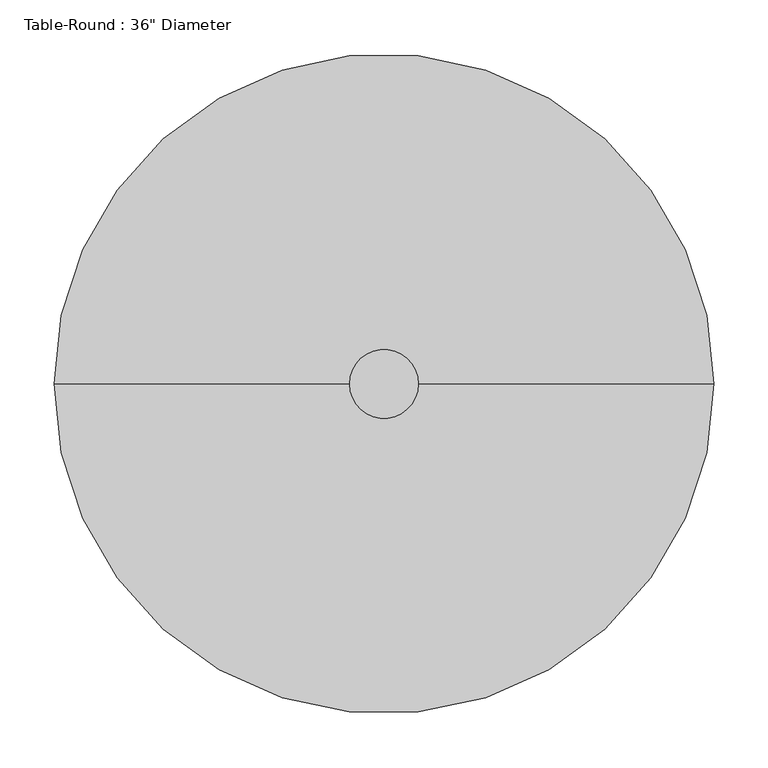
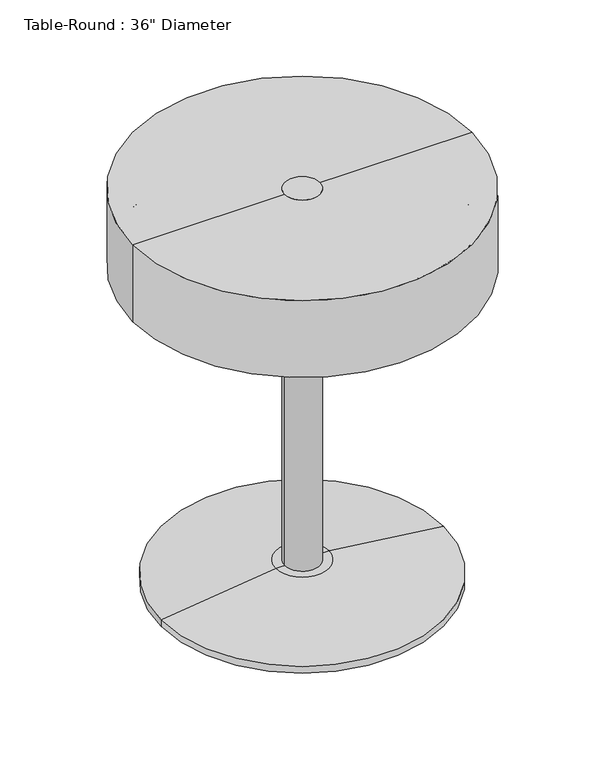
"""IFC4 building model written with IfcOpenShell, lengths in millimetres: furniture geometry."""

from ifc_helpers import new_model, si_unit, point, frame, origin, origin_2d, place, context, project, spatial, polyline, circle_curve, ellipse_curve, trimmed, segment, composite_curve, outline, extrude, source, transform, mapped, element, save
from ifc_brep_helpers import plane_surface, cylinder_surface, revolved_surface, advanced_brep


def furniture_3250926c(model_context):
    return source(origin(), model_context, "Body", "SolidModel", [
        extrude(outline(composite_curve([segment(trimmed(circle_curve(origin_2d(), 31.75), [point((-31.75, 0.0))], [point((31.75, 0.0))], False, "CARTESIAN"), True, "CONTINUOUS"), segment(trimmed(circle_curve(origin_2d(), 31.75), [point((31.75, 0.0))], [point((-31.75, 0.0))], False, "CARTESIAN"), True, "CONTINUOUS")], self_intersect=False)), frame((0.0, 0.0, 38.1), z_axis=(0.0, 0.0, 1.0), x_axis=(1.0, 0.0, 0.0)), (0.0, 0.0, 1.0), 704.85),
        advanced_brep(
        [(304.8, 0.0, 742.95), (-304.8, 0.0, 742.95), (0.0, 0.0, 742.95), (0.0, 0.0, 609.6), (-262.9011364, 0.0, 609.6), (262.9011364, 0.0, 609.6), (-299.5526659, 0.0, 603.1373465), (299.5526659, 0.0, 603.1373465), (-304.8, 0.0, 596.8838172), (304.8, 0.0, 596.8838172)],
        [
            (0, 1, circle_curve(frame((0.0, 0.0, 742.95), z_axis=(0.0, 0.0, 1.0), x_axis=(-1.0, 0.0, 0.0)), 304.8)),
            (1, 2),
            (2, 0),
            (1, 0, circle_curve(frame((0.0, 0.0, 742.95), z_axis=(0.0, 0.0, 1.0), x_axis=(-1.0, 0.0, 0.0)), 304.8)),
            (3, 4),
            (4, 5, circle_curve(frame((0.0, 0.0, 609.6), z_axis=(0.0, 0.0, -1.0), x_axis=(-1.0, 0.0, 0.0)), 262.9011364)),
            (5, 3),
            (5, 4, circle_curve(frame((0.0, 0.0, 609.6), z_axis=(0.0, 0.0, -1.0), x_axis=(-1.0, 0.0, 0.0)), 262.9011364)),
            (4, 6),
            (6, 7, circle_curve(frame((0.0, 0.0, 603.1373465), z_axis=(0.0, 0.0, -1.0), x_axis=(-1.0, 0.0, 0.0)), 299.5526659)),
            (7, 5),
            (7, 6, circle_curve(frame((0.0, 0.0, 603.1373465), z_axis=(0.0, 0.0, -1.0), x_axis=(-1.0, 0.0, 0.0)), 299.5526659)),
            (6, 8, circle_curve(frame((-298.45, 0.0, 596.8838172), z_axis=(0.0, -1.0, 0.0), x_axis=(1.0, 0.0, 0.0)), 6.35)),
            (8, 9, circle_curve(frame((0.0, 0.0, 596.8838172), z_axis=(0.0, 0.0, -1.0), x_axis=(-1.0, 0.0, 0.0)), 304.8)),
            (9, 7, circle_curve(frame((298.45, 0.0, 596.8838172), z_axis=(0.0, -1.0, 0.0), x_axis=(-1.0, 0.0, 0.0)), 6.35)),
            (9, 8, circle_curve(frame((0.0, 0.0, 596.8838172), z_axis=(0.0, 0.0, -1.0), x_axis=(-1.0, 0.0, 0.0)), 304.8)),
            (8, 1),
            (0, 9),
        ],
        [
            plane_surface(frame((0.0, 0.0, 742.95), z_axis=(0.0, 0.0, 1.0), x_axis=(-1.0, 0.0, 0.0))),
            plane_surface(frame((0.0, 0.0, 609.6), z_axis=(0.0, 0.0, -1.0), x_axis=(-1.0, 0.0, 0.0))),
            revolved_surface(polyline([(-299.5526659, 0.0, 603.1373465), (-262.9011364, 0.0, 609.6)]), (0.0, 0.0, 685.8), (0.0, 0.0, -1.0)),
            revolved_surface(trimmed(ellipse_curve(frame((-298.45, 0.0, 596.8838172), z_axis=(0.0, 1.0, 0.0), x_axis=(1.0, 0.0, 0.0)), 6.35, 6.35), [point((-304.8, 0.0, 596.8838172))], [point((-299.5526659, 0.0, 603.1373465))], True, "CARTESIAN"), (0.0, 0.0, 685.8), (0.0, 0.0, -1.0)),
            cylinder_surface(frame((0.0, 0.0, 685.8), z_axis=(0.0, 0.0, -1.0), x_axis=(-1.0, 0.0, 0.0)), 304.8),
        ],
        [
            (0, [[1, 2, 3]]),
            (0, [[4, -3, -2]]),
            (1, [[5, 6, 7]]),
            (1, [[-7, 8, -5]]),
            (2, [[-6, 9, 10, 11]]),
            (2, [[-8, -11, 12, -9]]),
            (3, [[-10, 13, 14, 15]]),
            (3, [[-12, -15, 16, -13]]),
            (4, [[-14, 17, -1, 18]]),
            (4, [[-16, -18, -4, -17]]),
        ],
    ),
        advanced_brep(
        [(0.0, 0.0, 0.0), (-254.0, 0.0, 0.0), (254.0, 0.0, 0.0), (47.625, 0.0, 38.1), (-47.625, 0.0, 38.1), (0.0, 0.0, 38.1), (254.0, 0.0, 12.7), (-254.0, 0.0, 12.7)],
        [
            (0, 1),
            (1, 2, circle_curve(frame((0.0, 0.0, 0.0), z_axis=(0.0, 0.0, -1.0), x_axis=(-1.0, 0.0, 0.0)), 254.0)),
            (2, 0),
            (2, 1, circle_curve(frame((0.0, 0.0, 0.0), z_axis=(0.0, 0.0, -1.0), x_axis=(-1.0, 0.0, 0.0)), 254.0)),
            (3, 4, circle_curve(frame((0.0, 0.0, 38.1), z_axis=(0.0, 0.0, 1.0), x_axis=(-1.0, 0.0, 0.0)), 47.625)),
            (4, 5),
            (5, 3),
            (4, 3, circle_curve(frame((0.0, 0.0, 38.1), z_axis=(0.0, 0.0, 1.0), x_axis=(-1.0, 0.0, 0.0)), 47.625)),
            (6, 7, circle_curve(frame((0.0, 0.0, 12.7), z_axis=(0.0, 0.0, 1.0), x_axis=(-1.0, 0.0, 0.0)), 254.0)),
            (7, 4),
            (3, 6),
            (7, 6, circle_curve(frame((0.0, 0.0, 12.7), z_axis=(0.0, 0.0, 1.0), x_axis=(-1.0, 0.0, 0.0)), 254.0)),
            (1, 7),
            (6, 2),
        ],
        [
            plane_surface(frame((0.0, 0.0, 0.0), z_axis=(0.0, 0.0, -1.0), x_axis=(-1.0, 0.0, 0.0))),
            plane_surface(frame((0.0, 0.0, 38.1), z_axis=(0.0, 0.0, 1.0), x_axis=(-1.0, 0.0, 0.0))),
            revolved_surface(polyline([(-47.625, 0.0, 38.1), (-254.0, 0.0, 12.7)]), (0.0, 0.0, 215.9), (0.0, 0.0, -1.0)),
            cylinder_surface(frame((0.0, 0.0, 215.9), z_axis=(0.0, 0.0, -1.0), x_axis=(-1.0, 0.0, 0.0)), 254.0),
        ],
        [
            (0, [[1, 2, 3]]),
            (0, [[-3, 4, -1]]),
            (1, [[5, 6, 7]]),
            (1, [[8, -7, -6]]),
            (2, [[9, 10, -5, 11]]),
            (2, [[12, -11, -8, -10]]),
            (3, [[-2, 13, -9, 14]]),
            (3, [[-4, -14, -12, -13]]),
        ],
    ),
    ])


if __name__ == "__main__":
    model = new_model("IFC4")
    model_context = context("Model", 3, world=origin())
    ifc_project = project(units=[si_unit("LENGTHUNIT", "METRE", prefix="MILLI")], contexts=[model_context])
    site = spatial("IfcSite", under=ifc_project)
    building = spatial("IfcBuilding", under=site)
    placement = place(None, origin())
    furniture_shape = furniture_3250926c(model_context)
    element("IfcFurniture", 1, ObjectType="Table-Round : 36\" Diameter", at=placement, inside=building, context=model_context, shape_type="MappedRepresentation", body=[
        mapped(furniture_shape, transform((0.0, 0.0, 0.0), x_axis=(1.0, 0.0, 0.0), y_axis=(0.0, 1.0, 0.0), z_axis=(0.0, 0.0, 1.0))),
    ])
    save(model, "model.ifc")

# Revit data of these elements
# Type "Table-Round : 36\" Diameter"
#   Assembly Code = "E2020200"
#   Base Radius = 0' - 10"
#   Height = 2' - 0"
#   Radius = 1' - 0"
#   Base Material = Steel, Chrome Plated
#   Top Material = Birch
#   Default Elevation = 0
# Element 1 (IfcFurniture, "Table-Round : 36\" Diameter")
#   Materials on its faces: "Steel, Chrome Plated", "Birch"
# Materials
#   "Steel, Chrome Plated": class "Metal", colour RGB 17 17 17, transparency 0, Description = "Chromiuim plated steel", Cost = 0
#   "Birch": class "Wood", colour RGB 210 159 95, transparency 0, Description = "Betula Alleghaniensis", Cost = 0
